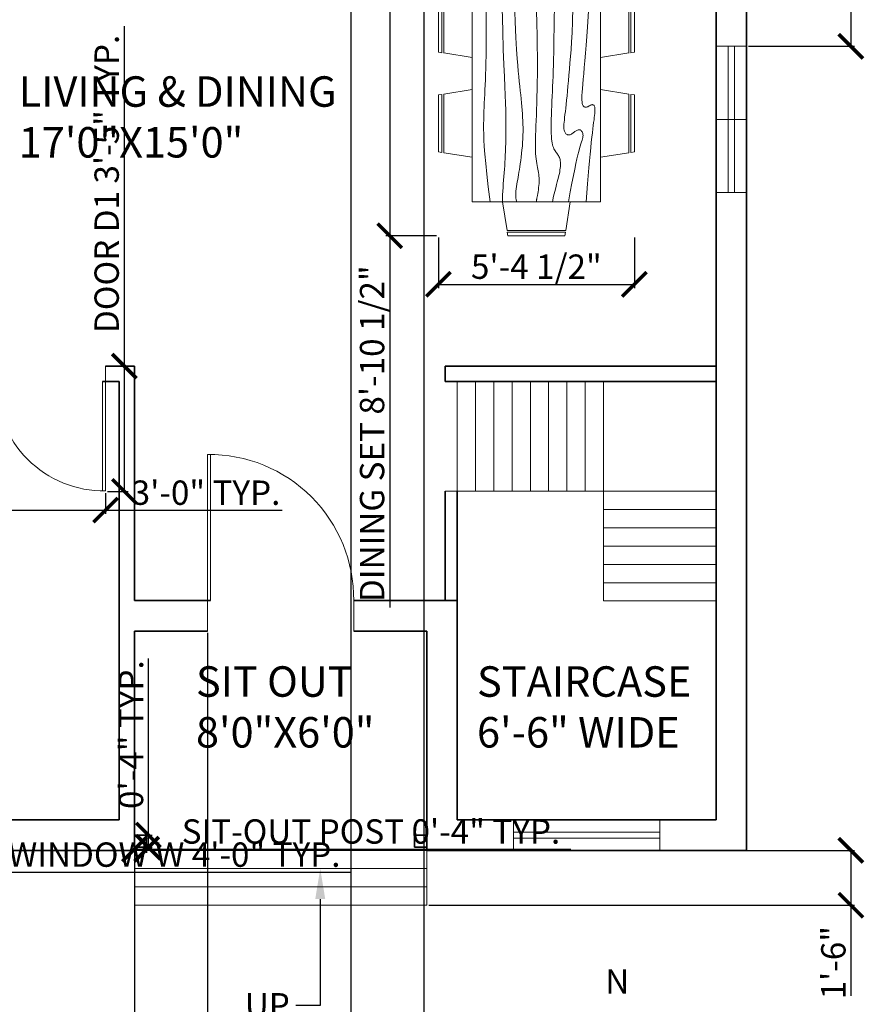
# Model space of a CAD drawing. Units: inches. Extents: x 21865 to 22885, y 36660 to 37408.
# Tile 3 of 6: x 22052 to 22329, y 36833 to 37157. Entities that reach past the tile are written whole.
import ezdxf
from ezdxf import colors
from ezdxf.entities.mleader import LeaderData, LeaderLine
from ezdxf.math import Vec2, Vec3

# ---------------------------------------------------------------- set-up
doc = ezdxf.new("R2010")
doc.units = ezdxf.units.IN
for name, color, linetype, lineweight in [('A-ANNO-DIMS', 2, 'Continuous', 18), ('A-ANNO-SYMB', 7, 'Continuous', 18), ('A-ANNO-TEXT', 7, 'Continuous', 18), ('A-AREA-IDEN', 7, 'Continuous', 20), ('A-COLS', 7, 'Continuous', 35), ('A-DOOR', 3, 'Continuous', 20), ('A-FLOR-STRS', 7, 'Continuous', 20), ('A-FURN', 8, 'Continuous', 18), ('A-GLAZ', 4, 'Continuous', 18), ('A-WALL', 7, 'Continuous', 35)]:
    doc.layers.add(name, color=color, linetype=linetype, lineweight=lineweight)
doc.styles.get("Standard").update_dxf_attribs({"font": 'arial.ttf'})
doc.dimstyles.new('ISO-25', dxfattribs={"dimtxt": 8, "dimasz": 8, "dimexe": 1.25, "dimexo": 0.625, "dimtad": 1, "dimlunit": 3, "dimtxsty": 'Standard', "dimblk": 'ARCHTICK', "dimcen": 2.5, "dimclrd": 4, "dimclre": 5, "dimclrt": 1, "dimadec": 0, "dimazin": 0, "dimtfac": 1, "dimtmove": 0, "dimatfit": 3, "dimfxl": 1, "dimarcsym": 0})

# ---------------------------------------------------------------- blocks, each defined once
blk = doc.blocks.new('Dining Set - 36 x 72 in.')
for p, q in [((-22.2343, 26.00059), (-23.4847, 17.99762)), ((-22.2304, 26), (-5.7608, 26)), ((-22, 27.5), (-22.1562, 26.50042)), ((-5.8416, 26.5), (-22.1534, 26.5)), ((-22, 27.5), (-6, 27.5)), ((-5.8437, 26.49966), (-6, 27.5)), ((-4.5152, 17.99762), (-5.7655, 25.99926)), ((5.7657, 26.00059), (4.5153, 17.99762)), ((5.7696, 26), (22.2392, 26)), ((6, 27.5), (5.8438, 26.50042)), ((22.1584, 26.5), (5.8466, 26.5)), ((6, 27.5), (22, 27.5)), ((22.1563, 26.49966), (22, 27.5)), ((23.4848, 17.99762), (22.2345, 25.99926)), ((36, 18), (-36, 18)), ((-36, 18), (-36, -18)), ((36, -18), (36, 18)), ((-44.0006, 8.23428), (-35.9976, 9.48474)), ((44.0006, 8.23428), (35.9976, 9.48474)), ((-45.5, 8), (-44.5004, 8.15617)), ((-45.5, 8), (-45.5, -8)), ((-44.5, -8.15843), (-44.5, 8.15338)), ((-44, 8.23041), (-44, -8.23915)), ((44, 8.23041), (44, -8.23915)), ((44.5, -8.15843), (44.5, 8.15338)), ((45.5, 8), (44.5005, 8.15617)), ((45.5, 8), (45.5, -8)), ((-44.4997, -8.15631), (-45.5, -8)), ((-35.9976, -9.48476), (-43.9993, -8.2345)), ((35.9976, -9.48476), (43.9993, -8.2345)), ((44.4997, -8.15631), (45.5, -8)), ((-36, -18), (36, -18)), ((-22.2343, -26.0006), (-23.4847, -17.99762)), ((-4.5152, -17.99762), (-5.7655, -25.99928)), ((5.7657, -26.0006), (4.5153, -17.99762)), ((23.4848, -17.99762), (22.2345, -25.99928)), ((-22.2304, -26), (-5.7608, -26)), ((-22, -27.5), (-22.1562, -26.50044)), ((-5.8416, -26.5), (-22.1534, -26.5)), ((-22, -27.5), (-6, -27.5)), ((-5.8437, -26.49967), (-6, -27.5)), ((5.7696, -26), (22.2392, -26)), ((6, -27.5), (5.8438, -26.50044)), ((22.1584, -26.5), (5.8466, -26.5)), ((6, -27.5), (22, -27.5)), ((22.1563, -26.49967), (22, -27.5))]:
    blk.add_line(p, q)
for points in [[(-36, 15), (-31.1772, 14.97754), (-26.8079, 14.91406), (-22.8538, 14.81543), (-19.276, 14.6875), (-16.0362, 14.53613), (-13.0957, 14.36718), (-10.4159, 14.18652), (-7.9583, 14), (-5.6904, 13.81315), (-3.6035, 13.63021), (-1.6954, 13.45508), (0.0365, 13.29166), (1.5945, 13.14388), (2.9811, 13.01562), (4.1988, 12.9108), (5.25, 12.83333), (6.1393, 12.78613), (6.8802, 12.76823), (7.4883, 12.77767), (7.9792, 12.8125), (8.3685, 12.87077), (8.6719, 12.95052), (8.9049, 13.0498), (9.0833, 13.16666), (9.2205, 13.29899), (9.3216, 13.44401), (9.3895, 13.59879), (9.4271, 13.76041), (9.4373, 13.92594), (9.4232, 14.09245), (9.3875, 14.257), (9.3333, 14.41666), (9.2638, 14.56917), (9.1836, 14.71484), (9.0975, 14.85465), (9.0104, 14.98958), (8.9272, 15.1206), (8.8529, 15.2487), (8.7922, 15.37483), (8.75, 15.5), (8.7305, 15.62467), (8.7344, 15.74739), (8.7617, 15.86621), (8.8125, 15.97916), (8.8867, 16.08431), (8.9844, 16.17968), (9.1055, 16.26334), (9.25, 16.33333), (9.4189, 16.38802), (9.6172, 16.42708), (9.8506, 16.45052), (10.125, 16.45833), (10.4463, 16.45052), (10.8203, 16.42708), (11.2529, 16.38802), (11.75, 16.33333), (12.3184, 16.26318), (12.9694, 16.17838), (13.7151, 16.07991), (14.5677, 15.96875), (15.5395, 15.84586), (16.6426, 15.71224), (17.8893, 15.56884), (19.2917, 15.41666), (20.859, 15.25667), (22.5879, 15.08984), (24.4721, 14.91715), (26.5052, 14.73958), (28.6809, 14.5581), (30.9929, 14.3737), (33.4347, 14.18733), (36, 14)], [(-36, 10), (-28.9766, 10.14274), (-23.1725, 10.20442), (-18.4241, 10.19775), (-14.5677, 10.13541), (-11.4399, 10.03011), (-8.877, 9.89453), (-6.7154, 9.74137), (-4.7917, 9.58333), (-2.9698, 9.43082), (-1.2246, 9.28515), (0.4415, 9.14534), (2.026, 9.01041), (3.5266, 8.87939), (4.9408, 8.7513), (6.266, 8.62516), (7.5, 8.5), (8.6411, 8.37549), (9.6914, 8.2539), (10.6538, 8.13818), (11.5312, 8.03125), (12.3267, 7.93603), (13.043, 7.85547), (13.6831, 7.79248), (14.25, 7.75), (14.7471, 7.7303), (15.1797, 7.73307), (15.5537, 7.75732), (15.875, 7.80208), (16.1494, 7.86637), (16.3828, 7.94922), (16.5811, 8.04964), (16.75, 8.16666), (16.8944, 8.29915), (17.0143, 8.44531), (17.1089, 8.60319), (17.1771, 8.77083), (17.218, 8.94629), (17.2305, 9.1276), (17.2137, 9.31282), (17.1667, 9.5), (17.0895, 9.6875), (16.987, 9.875), (16.8649, 10.0625), (16.7292, 10.25), (16.5856, 10.4375), (16.4401, 10.625), (16.2985, 10.8125), (16.1667, 11), (16.05, 11.18733), (15.9518, 11.3737), (15.8752, 11.5581), (15.8229, 11.73958), (15.798, 11.91715), (15.8034, 12.08984), (15.842, 12.25667), (15.9167, 12.41666), (16.0295, 12.56836), (16.1784, 12.70833), (16.3605, 12.83268), (16.5729, 12.9375), (16.8127, 13.01888), (17.0768, 13.07291), (17.3625, 13.0957), (17.6667, 13.08333), (17.9894, 13.03312), (18.3418, 12.94726), (18.7382, 12.82918), (19.1927, 12.68229), (19.7195, 12.51001), (20.3327, 12.31575), (21.0465, 12.10294), (21.875, 11.875), (22.8357, 11.63354), (23.959, 11.37304), (25.2786, 11.08618), (26.8282, 10.76562), (28.6414, 10.40405), (30.752, 9.99414), (33.1936, 9.52856), (36, 9)], [(-36, 5.5), (-30.7157, 5.3348), (-26.069, 5.20963), (-21.9946, 5.11767), (-18.4271, 5.05208), (-15.3009, 5.00602), (-12.5508, 4.97265), (-10.1112, 4.94515), (-7.9167, 4.91666), (-5.909, 4.88167), (-4.0586, 4.83984), (-2.3429, 4.79215), (-0.7396, 4.73958), (0.7739, 4.6831), (2.22, 4.6237), (3.6213, 4.56233), (5, 4.5), (6.373, 4.43782), (7.7344, 4.3776), (9.0723, 4.32129), (10.375, 4.27083), (11.6309, 4.22819), (12.8281, 4.19531), (13.9551, 4.17415), (15, 4.16666), (15.954, 4.17448), (16.819, 4.19791), (17.6001, 4.23698), (18.3021, 4.29166), (18.9299, 4.36198), (19.4883, 4.44791), (19.9823, 4.54948), (20.4167, 4.66666), (20.7969, 4.79899), (21.1302, 4.94401), (21.4245, 5.09879), (21.6875, 5.26041), (21.9271, 5.42594), (22.1511, 5.59245), (22.3672, 5.757), (22.5834, 5.91666), (22.8065, 6.06868), (23.0404, 6.21093), (23.2879, 6.34147), (23.5521, 6.45833), (23.8358, 6.55957), (24.142, 6.64323), (24.4735, 6.70735), (24.8334, 6.75), (25.2235, 6.76969), (25.642, 6.76692), (26.0858, 6.74267), (26.5521, 6.69791), (27.0379, 6.63362), (27.5404, 6.55078), (28.0565, 6.45036), (28.5834, 6.33333), (29.1242, 6.19987), (29.7071, 6.04687), (30.3661, 5.87044), (31.1354, 5.66666), (32.0493, 5.43164), (33.142, 5.16146), (34.4475, 4.85221), (36, 4.5)], [(-36, -1), (-30.7915, -0.6591), (-26.0195, -0.38216), (-21.6519, -0.16284), (-17.6563, 0.00521), (-14.0005, 0.12833), (-10.6523, 0.21289), (-7.5796, 0.26522), (-4.75, 0.29166), (-2.134, 0.29793), (0.2878, 0.28711), (2.5317, 0.26163), (4.6146, 0.22396), (6.5529, 0.17651), (8.3633, 0.12174), (10.0623, 0.06209), (11.6667, 0), (13.1899, -0.06201), (14.6341, -0.1211), (15.9982, -0.17432), (17.2813, -0.21875), (18.4823, -0.25147), (19.6003, -0.26953), (20.6343, -0.27002), (21.5834, -0.25), (22.4481, -0.20768), (23.2357, -0.14584), (23.9549, -0.06836), (24.6146, 0.02083), (25.2235, 0.11784), (25.7904, 0.21875), (26.3241, 0.31966), (26.8334, 0.41666), (27.3265, 0.50618), (27.8099, 0.58593), (28.2894, 0.65397), (28.7709, 0.70833), (29.2601, 0.74707), (29.763, 0.76823), (30.2855, 0.76985), (30.8334, 0.75), (31.4088, 0.70784), (31.9994, 0.64713), (32.589, 0.57275), (33.1615, 0.48958), (33.7008, 0.4025), (34.1908, 0.3164), (34.6153, 0.23616), (34.9584, 0.16666), (35.2099, 0.11165), (35.3848, 0.07031), (35.504, 0.04069), (35.5886, 0.02083), (35.6594, 0.00879), (35.7377, 0.0026), (35.8442, 0.00032), (36, 0)], [(-36, -6.5), (-27.1843, -6.31267), (-20.084, -6.1263), (-14.469, -5.9419), (-10.1094, -5.76042), (-6.7752, -5.58285), (-4.2363, -5.41016), (-2.2629, -5.24333), (-0.625, -5.08334), (0.8708, -4.93099), (2.2715, -4.78646), (3.5872, -4.64974), (4.8281, -4.52084), (6.0046, -4.39974), (7.127, -4.28646), (8.2053, -4.18099), (9.25, -4.08334), (10.2705, -3.99382), (11.2734, -3.91407), (12.2647, -3.84603), (13.25, -3.79167), (14.2354, -3.75293), (15.2266, -3.73177), (16.2295, -3.73015), (17.25, -3.75), (18.2912, -3.79248), (19.3451, -3.85547), (20.4009, -3.93604), (21.4479, -4.03125), (22.4754, -4.13819), (23.4727, -4.25391), (24.4289, -4.37549), (25.3334, -4.5), (26.1785, -4.62492), (26.9694, -4.74935), (27.7145, -4.87281), (28.4219, -4.99479), (29.1, -5.11483), (29.7572, -5.23242), (30.4016, -5.34709), (31.0417, -5.45834), (31.6837, -5.56437), (32.3262, -5.65821), (32.9658, -5.73153), (33.599, -5.77604), (34.2224, -5.78345), (34.8327, -5.74545), (35.4264, -5.65373), (36, -5.5)], [(-36, -10), (-26.4022, -9.81299), (-18.4675, -9.62891), (-11.9839, -9.45069), (-6.7396, -9.28125), (-2.5226, -9.12354), (0.8789, -8.98047), (3.6769, -8.85498), (6.0833, -8.75), (8.2767, -8.66765), (10.3021, -8.60677), (12.1712, -8.56543), (13.8958, -8.54167), (15.4876, -8.53353), (16.9583, -8.53907), (18.3197, -8.55632), (19.5834, -8.58334), (20.7616, -8.61841), (21.8685, -8.66081), (22.9188, -8.71004), (23.9271, -8.76563), (24.9081, -8.82707), (25.8763, -8.89388), (26.8465, -8.96558), (27.8334, -9.04167), (28.8474, -9.12118), (29.8828, -9.20117), (30.93, -9.27824), (31.9792, -9.34896), (33.0205, -9.40991), (34.0443, -9.45768), (35.0407, -9.48885), (36, -9.5)], [(-36, -14.5), (-30.0881, -14.33513), (-25.0332, -14.21224), (-20.7312, -14.12647), (-17.0781, -14.07292), (-13.97, -14.04671), (-11.3027, -14.04297), (-8.9724, -14.05681), (-6.875, -14.08334), (-4.9224, -14.11833), (-3.0905, -14.16016), (-1.3709, -14.20785), (0.2448, -14.26042), (1.7647, -14.3169), (3.1973, -14.3763), (4.5507, -14.43767), (5.8333, -14.5), (7.0554, -14.5621), (8.235, -14.62175), (9.3922, -14.67652), (10.5469, -14.72396), (11.7192, -14.76164), (12.929, -14.78711), (14.1965, -14.79794), (15.5417, -14.79167), (16.9933, -14.76424), (18.6152, -14.70508), (20.4804, -14.60197), (22.6615, -14.44271), (25.2312, -14.21509), (28.2624, -13.9069), (31.8277, -13.50594), (36, -13)]]:
    blk.add_lwpolyline(points)
blk = doc.blocks.new('WIN-W-48-PLAN')
for p, q in [((0, 0), (0, 10)), ((48, 0), (48, 10)), ((48, 6), (0, 6)), ((48, 4), (0, 4))]:
    blk.add_line(p, q)
blk = doc.blocks.new('DOOR-D1-36-PLAN')
for p, q in [((0, 36), (0, 41)), ((36, 36), (36, 41)), ((35, 36), (35, 0)), ((36, 36), (36, 0))]:
    blk.add_line(p, q)
blk.add_arc((35.5, 35.5), 35.5, 179.1931, 270.8069)
blk = doc.blocks.new('POST-SITOUT-4')
for p, q in [((4, 4), (0, 4)), ((4, 0), (4, 4)), ((0, 0), (2, 0)), ((2, 0), (4, 0))]:
    blk.add_line(p, q)
blk = doc.blocks.new('_ArchTick')
at = {"color": 0, "linetype": 'ByBlock', "const_width": 0.15}
blk.add_lwpolyline([(-0.5, -0.5), (0.5, 0.5)], dxfattribs=at)
blk = doc.blocks.new('*D30')
at = {"layer": 'A-ANNO-DIMS', "color": 5, "lineweight": -2, "transparency": 16777216}
for p, q in [((21988.43, 36883.31), (21988.43, 36875.48)), ((22036.43, 36883.31), (22036.43, 36875.48))]:
    blk.add_line(p, q, dxfattribs=at)
at = {"layer": 'A-ANNO-DIMS', "color": 4, "lineweight": -2, "transparency": 16777216}
for p, q in [((21988.43, 36876.73), (22036.43, 36876.73)), ((22036.43, 36876.73), (22160.57, 36876.73))]:
    blk.add_line(p, q, dxfattribs=at)
at = {"layer": 'Defpoints', "color": 0, "transparency": 16777216}
for p in [(21988.43, 36883.93), (22036.43, 36883.93), (22036.43, 36876.73)]:
    blk.add_point(p, dxfattribs=at)
at = {"layer": 'A-ANNO-DIMS', "color": 4, "lineweight": -2, "transparency": 16777216, "xscale": 8, "yscale": 8, "zscale": 8, "rotation": 180}
blk.add_blockref('_ArchTick', (21988.43, 36876.73), dxfattribs=at)
at = {"layer": 'A-ANNO-DIMS', "color": 4, "lineweight": -2, "transparency": 16777216, "xscale": 8, "yscale": 8, "zscale": 8}
blk.add_blockref('_ArchTick', (22036.43, 36876.73), dxfattribs=at)
at = {"layer": 'A-ANNO-DIMS', "color": 1, "transparency": 16777216, "insert": (22102.5, 36881.5), "char_height": 8, "attachment_point": 5}
blk.add_mtext('WINDOW W 4\'-0" TYP.', dxfattribs=at)
blk = doc.blocks.new('*D36')
at = {"layer": 'A-ANNO-DIMS', "color": 4, "lineweight": -2, "transparency": 16777216}
for p, q in [((22086.1, 37042.93), (22086.1, 37154.57)), ((22086.1, 37001.8), (22086.1, 37042.93))]:
    blk.add_line(p, q, dxfattribs=at)
at = {"layer": 'A-ANNO-DIMS', "color": 5, "lineweight": -2, "transparency": 16777216}
for p, q in [((22080.55, 37042.93), (22087.35, 37042.93)), ((22080.55, 37001.8), (22087.35, 37001.8))]:
    blk.add_line(p, q, dxfattribs=at)
at = {"layer": 'Defpoints', "color": 0, "transparency": 16777216}
for p in [(22079.93, 37042.93), (22086.1, 37042.93), (22079.93, 37001.8)]:
    blk.add_point(p, dxfattribs=at)
at = {"layer": 'A-ANNO-DIMS', "color": 4, "lineweight": -2, "transparency": 16777216, "xscale": 8, "yscale": 8, "zscale": 8}
for p, rotation in [((22086.1, 37042.93), 90), ((22086.1, 37001.8), 270)]:
    blk.add_blockref('_ArchTick', p, dxfattribs=dict(at, rotation=rotation))
at = {"layer": 'A-ANNO-DIMS', "color": 1, "transparency": 16777216, "insert": (22081.33, 37102.75), "char_height": 8, "attachment_point": 5, "rotation": 90}
blk.add_mtext('DOOR D1 3\'-5" TYP.', dxfattribs=at)
blk = doc.blocks.new('*D37')
at = {"layer": 'A-ANNO-DIMS', "color": 5, "lineweight": -2, "transparency": 16777216}
for p, q in [((22043.79, 37001.17), (22043.79, 36994.38)), ((22079.93, 37001.17), (22079.93, 36994.38))]:
    blk.add_line(p, q, dxfattribs=at)
at = {"layer": 'A-ANNO-DIMS', "color": 4, "lineweight": -2, "transparency": 16777216}
for p, q in [((22043.79, 36995.63), (22079.93, 36995.63)), ((22079.93, 36995.63), (22137.94, 36995.63))]:
    blk.add_line(p, q, dxfattribs=at)
at = {"layer": 'Defpoints', "color": 0, "transparency": 16777216}
for p in [(22043.79, 37001.8), (22079.93, 37001.8), (22079.93, 36995.63)]:
    blk.add_point(p, dxfattribs=at)
at = {"layer": 'A-ANNO-DIMS', "color": 4, "lineweight": -2, "transparency": 16777216, "xscale": 8, "yscale": 8, "zscale": 8, "rotation": 180}
blk.add_blockref('_ArchTick', (22043.79, 36995.63), dxfattribs=at)
at = {"layer": 'A-ANNO-DIMS', "color": 4, "lineweight": -2, "transparency": 16777216, "xscale": 8, "yscale": 8, "zscale": 8}
blk.add_blockref('_ArchTick', (22079.93, 36995.63), dxfattribs=at)
at = {"layer": 'A-ANNO-DIMS', "color": 1, "transparency": 16777216, "insert": (22112.93, 37000.34), "char_height": 8, "attachment_point": 5}
blk.add_mtext('3\'-0" TYP.', dxfattribs=at)
blk = doc.blocks.new('*D38')
at = {"layer": 'A-ANNO-DIMS', "color": 4, "lineweight": -2, "transparency": 16777216}
for p, q in [((22089.43, 36884.34), (22093.43, 36884.34)), ((22093.43, 36884.34), (22232.74, 36884.34))]:
    blk.add_line(p, q, dxfattribs=at)
at = {"layer": 'A-ANNO-DIMS', "color": 5, "lineweight": -2, "transparency": 16777216}
for p, q in [((22089.43, 36884.31), (22089.43, 36883.09)), ((22093.43, 36884.31), (22093.43, 36883.09))]:
    blk.add_line(p, q, dxfattribs=at)
at = {"layer": 'Defpoints', "color": 0, "transparency": 16777216}
for p in [(22089.43, 36884.94), (22093.43, 36884.94), (22093.43, 36884.34)]:
    blk.add_point(p, dxfattribs=at)
at = {"layer": 'A-ANNO-DIMS', "color": 4, "lineweight": -2, "transparency": 16777216, "xscale": 8, "yscale": 8, "zscale": 8, "rotation": 180}
blk.add_blockref('_ArchTick', (22089.43, 36884.34), dxfattribs=at)
at = {"layer": 'A-ANNO-DIMS', "color": 4, "lineweight": -2, "transparency": 16777216, "xscale": 8, "yscale": 8, "zscale": 8}
blk.add_blockref('_ArchTick', (22093.43, 36884.34), dxfattribs=at)
at = {"layer": 'A-ANNO-DIMS', "color": 1, "transparency": 16777216, "insert": (22167.09, 36889.1), "char_height": 8, "attachment_point": 5}
blk.add_mtext('SIT-OUT POST 0\'-4" TYP.', dxfattribs=at)
blk = doc.blocks.new('*D39')
at = {"layer": 'A-ANNO-DIMS', "color": 4, "lineweight": -2, "transparency": 16777216}
for p, q in [((22094.03, 36888.94), (22094.03, 36946.95)), ((22094.03, 36884.94), (22094.03, 36888.94))]:
    blk.add_line(p, q, dxfattribs=at)
at = {"layer": 'A-ANNO-DIMS', "color": 5, "lineweight": -2, "transparency": 16777216}
for p, q in [((22094.05, 36888.94), (22095.28, 36888.94)), ((22094.05, 36884.94), (22095.28, 36884.94))]:
    blk.add_line(p, q, dxfattribs=at)
at = {"layer": 'Defpoints', "color": 0, "transparency": 16777216}
for p in [(22093.43, 36888.94), (22094.03, 36888.94), (22093.43, 36884.94)]:
    blk.add_point(p, dxfattribs=at)
at = {"layer": 'A-ANNO-DIMS', "color": 4, "lineweight": -2, "transparency": 16777216, "xscale": 8, "yscale": 8, "zscale": 8}
for p, rotation in [((22094.03, 36888.94), 90), ((22094.03, 36884.94), 270)]:
    blk.add_blockref('_ArchTick', p, dxfattribs=dict(at, rotation=rotation))
at = {"layer": 'A-ANNO-DIMS', "color": 1, "transparency": 16777216, "insert": (22089.32, 36921.94), "char_height": 8, "attachment_point": 5, "rotation": 90}
blk.add_mtext('0\'-4" TYP.', dxfattribs=at)
blk = doc.blocks.new('*D48')
at = {"layer": 'A-ANNO-DIMS', "color": 5, "lineweight": -2, "transparency": 16777216}
for p, q in [((22188.6, 37192.23), (22172.01, 37192.23)), ((22188.6, 37085.76), (22172.01, 37085.76))]:
    blk.add_line(p, q, dxfattribs=at)
at = {"layer": 'A-ANNO-DIMS', "color": 4, "lineweight": -2, "transparency": 16777216}
for p, q in [((22173.26, 37192.23), (22173.26, 37085.76)), ((22173.26, 37085.76), (22173.26, 36963.72))]:
    blk.add_line(p, q, dxfattribs=at)
at = {"layer": 'Defpoints', "color": 0, "transparency": 16777216}
for p in [(22189.23, 37192.23), (22173.26, 37085.76), (22189.23, 37085.76)]:
    blk.add_point(p, dxfattribs=at)
at = {"layer": 'A-ANNO-DIMS', "color": 4, "lineweight": -2, "transparency": 16777216, "xscale": 8, "yscale": 8, "zscale": 8}
for p, rotation in [((22173.26, 37192.23), 90), ((22173.26, 37085.76), 270)]:
    blk.add_blockref('_ArchTick', p, dxfattribs=dict(at, rotation=rotation))
at = {"layer": 'A-ANNO-DIMS', "color": 1, "transparency": 16777216, "insert": (22168.49, 37020.74), "char_height": 8, "attachment_point": 5, "rotation": 90}
blk.add_mtext('DINING SET 8\'-10 1/2"', dxfattribs=at)
blk = doc.blocks.new('*D49')
at = {"layer": 'A-ANNO-DIMS', "color": 5, "lineweight": -2, "transparency": 16777216}
for p, q in [((22189.23, 37085.13), (22189.23, 37068.53)), ((22253.58, 37085.13), (22253.58, 37068.53))]:
    blk.add_line(p, q, dxfattribs=at)
at = {"layer": 'A-ANNO-DIMS', "color": 4, "lineweight": -2, "transparency": 16777216}
blk.add_line((22189.23, 37069.78), (22253.58, 37069.78), dxfattribs=at)
at = {"layer": 'Defpoints', "color": 0, "transparency": 16777216}
for p in [(22189.23, 37085.76), (22253.58, 37085.76), (22253.58, 37069.78)]:
    blk.add_point(p, dxfattribs=at)
at = {"layer": 'A-ANNO-DIMS', "color": 4, "lineweight": -2, "transparency": 16777216, "xscale": 8, "yscale": 8, "zscale": 8, "rotation": 180}
blk.add_blockref('_ArchTick', (22189.23, 37069.78), dxfattribs=at)
at = {"layer": 'A-ANNO-DIMS', "color": 4, "lineweight": -2, "transparency": 16777216, "xscale": 8, "yscale": 8, "zscale": 8}
blk.add_blockref('_ArchTick', (22253.58, 37069.78), dxfattribs=at)
at = {"layer": 'A-ANNO-DIMS', "color": 1, "transparency": 16777216, "insert": (22221.4, 37074.55), "char_height": 8, "attachment_point": 5}
blk.add_mtext('5\'-4 1/2"', dxfattribs=at)
blk = doc.blocks.new('*D57')
at = {"layer": 'A-ANNO-DIMS', "color": 5, "lineweight": -2, "transparency": 16777216}
for p, q in [((22291.05, 37269.93), (22325.93, 37269.93)), ((22291.05, 37147.93), (22325.93, 37147.93))]:
    blk.add_line(p, q, dxfattribs=at)
at = {"layer": 'A-ANNO-DIMS', "color": 4, "lineweight": -2, "transparency": 16777216}
blk.add_line((22324.68, 37269.93), (22324.68, 37147.93), dxfattribs=at)
at = {"layer": 'Defpoints', "color": 0, "transparency": 16777216}
for p in [(22290.43, 37269.93), (22290.43, 37147.93), (22324.68, 37147.93)]:
    blk.add_point(p, dxfattribs=at)
at = {"layer": 'A-ANNO-DIMS', "color": 4, "lineweight": -2, "transparency": 16777216, "xscale": 8, "yscale": 8, "zscale": 8}
for p, rotation in [((22324.68, 37269.93), 90), ((22324.68, 37147.93), 270)]:
    blk.add_blockref('_ArchTick', p, dxfattribs=dict(at, rotation=rotation))
at = {"layer": 'A-ANNO-DIMS', "color": 1, "transparency": 16777216, "insert": (22319.97, 37208.93), "char_height": 8, "attachment_point": 5, "rotation": 90}
blk.add_mtext('10\'-2"', dxfattribs=at)
blk = doc.blocks.new('*D58')
at = {"layer": 'A-ANNO-DIMS', "color": 5, "lineweight": -2, "transparency": 16777216}
for p, q in [((22160.43, 37233.31), (22160.43, 36662.83)), ((22184.43, 37233.31), (22184.43, 36662.83))]:
    blk.add_line(p, q, dxfattribs=at)
at = {"layer": 'A-ANNO-DIMS', "color": 4, "lineweight": -2, "transparency": 16777216}
blk.add_line((22160.43, 36664.08), (22184.43, 36664.08), dxfattribs=at)
at = {"layer": 'Defpoints', "color": 0, "transparency": 16777216}
for p in [(22160.43, 37233.93), (22184.43, 37233.93), (22184.43, 36664.08)]:
    blk.add_point(p, dxfattribs=at)
at = {"layer": 'A-ANNO-DIMS', "color": 4, "lineweight": -2, "transparency": 16777216, "xscale": 8, "yscale": 8, "zscale": 8, "rotation": 180}
blk.add_blockref('_ArchTick', (22160.43, 36664.08), dxfattribs=at)
at = {"layer": 'A-ANNO-DIMS', "color": 4, "lineweight": -2, "transparency": 16777216, "xscale": 8, "yscale": 8, "zscale": 8}
blk.add_blockref('_ArchTick', (22184.43, 36664.08), dxfattribs=at)
at = {"layer": 'A-ANNO-DIMS', "color": 1, "transparency": 16777216, "insert": (22172.43, 36668.79), "char_height": 8, "attachment_point": 5}
blk.add_mtext('2\'-0"', dxfattribs=at)
blk = doc.blocks.new('*D59')
at = {"layer": 'A-ANNO-DIMS', "color": 5, "lineweight": -2, "transparency": 16777216}
for p, q in [((22089.43, 36955.31), (22089.43, 36662.83)), ((22113.43, 36955.31), (22113.43, 36662.83))]:
    blk.add_line(p, q, dxfattribs=at)
at = {"layer": 'A-ANNO-DIMS', "color": 4, "lineweight": -2, "transparency": 16777216}
blk.add_line((22089.43, 36664.08), (22113.43, 36664.08), dxfattribs=at)
at = {"layer": 'Defpoints', "color": 0, "transparency": 16777216}
for p in [(22089.43, 36955.93), (22113.43, 36955.93), (22113.43, 36664.08)]:
    blk.add_point(p, dxfattribs=at)
at = {"layer": 'A-ANNO-DIMS', "color": 4, "lineweight": -2, "transparency": 16777216, "xscale": 8, "yscale": 8, "zscale": 8, "rotation": 180}
blk.add_blockref('_ArchTick', (22089.43, 36664.08), dxfattribs=at)
at = {"layer": 'A-ANNO-DIMS', "color": 4, "lineweight": -2, "transparency": 16777216, "xscale": 8, "yscale": 8, "zscale": 8}
blk.add_blockref('_ArchTick', (22113.43, 36664.08), dxfattribs=at)
at = {"layer": 'A-ANNO-DIMS', "color": 1, "transparency": 16777216, "insert": (22101.43, 36668.79), "char_height": 8, "attachment_point": 5}
blk.add_mtext('2\'-0"', dxfattribs=at)
blk = doc.blocks.new('*D60')
at = {"layer": 'A-ANNO-DIMS', "color": 5, "lineweight": -2, "transparency": 16777216}
for p, q in [((22186.05, 36883.93), (22325.93, 36883.93)), ((22186.05, 36865.93), (22325.93, 36865.93))]:
    blk.add_line(p, q, dxfattribs=at)
at = {"layer": 'A-ANNO-DIMS', "color": 4, "lineweight": -2, "transparency": 16777216}
for p, q in [((22324.68, 36883.93), (22324.68, 36865.93)), ((22324.68, 36865.93), (22324.68, 36836.17))]:
    blk.add_line(p, q, dxfattribs=at)
at = {"layer": 'Defpoints', "color": 0, "transparency": 16777216}
for p in [(22185.43, 36883.93), (22185.43, 36865.93), (22324.68, 36865.93)]:
    blk.add_point(p, dxfattribs=at)
at = {"layer": 'A-ANNO-DIMS', "color": 4, "lineweight": -2, "transparency": 16777216, "xscale": 8, "yscale": 8, "zscale": 8}
for p, rotation in [((22324.68, 36883.93), 90), ((22324.68, 36865.93), 270)]:
    blk.add_blockref('_ArchTick', p, dxfattribs=dict(at, rotation=rotation))
at = {"layer": 'A-ANNO-DIMS', "color": 1, "transparency": 16777216, "insert": (22319.97, 36847.05), "char_height": 8, "attachment_point": 5, "rotation": 90}
blk.add_mtext('1\'-6"', dxfattribs=at)

msp = doc.modelspace()

# ---------------------------------------------------------------- linework, layer by layer
at = {"layer": 'A-DOOR'}
for p, q in [((22113.43, 36965.931), (22113.43, 37013.931)), ((22114.43, 36965.931), (22114.43, 37013.931)), ((22113.43, 36955.931), (22113.43, 36965.931)), ((22161.43, 36955.931), (22161.43, 36965.931)), ((22161.43, 36965.931), (22161.43, 36965.931))]:
    msp.add_line(p, q, dxfattribs=at)
msp.add_arc((22113.93, 36966.431), 47.503, 359.39691, 90.60309, dxfattribs=at)
at = {"layer": 'A-FLOR-STRS'}
for p, q in [((22195.43, 37001.826), (22195.43, 37037.931)), ((22201.43, 37001.826), (22201.43, 37037.931)), ((22207.43, 37001.826), (22207.43, 37037.931)), ((22213.43, 37001.826), (22213.43, 37037.931)), ((22219.43, 37001.826), (22219.43, 37037.931)), ((22225.43, 37001.826), (22225.43, 37037.931)), ((22231.43, 37001.826), (22231.43, 37037.931)), ((22237.43, 37001.826), (22237.43, 37037.931)), ((22243.43, 37001.826), (22243.43, 37037.931)), ((22191.43, 37001.826), (22280.43, 37001.826)), ((22243.43, 37001.826), (22243.43, 36965.826)), ((22243.43, 36995.826), (22280.43, 36995.826)), ((22243.43, 36989.826), (22280.43, 36989.826)), ((22243.43, 36983.826), (22280.43, 36983.826)), ((22243.43, 36977.826), (22280.43, 36977.826)), ((22243.43, 36971.826), (22280.43, 36971.826)), ((22243.43, 36965.826), (22280.43, 36965.826)), ((22089.43, 36883.931), (22185.43, 36883.931)), ((22089.43, 36883.931), (22089.43, 36865.931)), ((22185.43, 36883.931), (22185.43, 36865.931)), ((22089.43, 36877.931), (22185.43, 36877.931)), ((22089.43, 36871.931), (22185.43, 36871.931)), ((22089.43, 36865.931), (22185.43, 36865.931))]:
    msp.add_line(p, q, dxfattribs=at)
at = {"layer": 'A-GLAZ'}
msp.add_line((22290.43, 37123.931), (22280.43, 37123.931), dxfattribs=at)
at = {"layer": 'A-WALL'}
for p, q in [((22290.43, 37363.931), (22290.43, 36883.931)), ((22280.43, 37229.931), (22280.43, 36893.931)), ((22089.43, 37042.931), (22079.93, 37042.931)), ((22089.43, 36965.931), (22089.43, 37042.931)), ((22280.43, 37042.931), (22191.43, 37042.931)), ((22191.43, 37037.931), (22191.43, 37042.931)), ((22084.43, 37037.931), (22078.93, 37037.931)), ((22084.43, 37037.931), (22078.93, 37037.931)), ((22084.43, 36893.931), (22084.43, 37037.931)), ((22280.43, 37037.931), (22191.43, 37037.931)), ((22191.43, 36965.931), (22191.43, 37001.826)), ((22191.43, 36965.931), (22191.43, 37001.826)), ((22195.43, 36975.931), (22195.43, 37001.826)), ((22195.43, 36893.931), (22195.43, 36975.931)), ((22114.43, 36965.931), (22089.43, 36965.931)), ((22195.43, 36965.931), (22161.43, 36965.931)), ((22089.43, 36883.931), (22089.43, 36955.931)), ((22113.43, 36955.931), (22089.43, 36955.931)), ((22185.43, 36955.931), (22161.43, 36955.931)), ((22185.43, 36883.931), (22185.43, 36955.931)), ((22084.43, 36893.931), (21940.43, 36893.931)), ((22280.43, 36893.931), (22195.43, 36893.931)), ((22089.43, 36883.931), (21930.43, 36883.931)), ((22290.43, 36883.931), (22185.43, 36883.931))]:
    msp.add_line(p, q, dxfattribs=at)

# ---------------------------------------------------------------- block references
at = {"layer": 'A-COLS'}
msp.add_blockref('POST-SITOUT-4', (22089.43, 36884.938), dxfattribs=at)
at = {"layer": 'A-COLS', "extrusion": (0, 0, -1), "zscale": -1}
msp.add_blockref('POST-SITOUT-4', (-22185.43, 36884.938), dxfattribs=at)
at = {"layer": 'A-DOOR'}
msp.add_blockref('DOOR-D1-36-PLAN', (22043.929, 37001.93), dxfattribs=at)
at = {"layer": 'A-FURN', "xscale": 1.170096591713225, "yscale": 1.170096591713225, "zscale": 1.170096591713225, "rotation": 270}
msp.add_blockref('Dining Set - 36 x 72 in.', (22221.405, 37138.995), dxfattribs=at)
at = {"layer": 'A-GLAZ', "rotation": 269.9999999999834}
msp.add_blockref('WIN-W-48-PLAN', (22280.429, 37147.931), dxfattribs=at)
at = {"layer": 'A-GLAZ'}
msp.add_blockref('WIN-W-48-PLAN', (22213.93, 36883.931), dxfattribs=at)

# ---------------------------------------------------------------- texts
at = {"layer": 'A-ANNO-SYMB', "insert": (22244.029, 36844.925), "char_height": 8, "width": 22.941, "attachment_point": 1}
msp.add_mtext('N', dxfattribs=at)
at = {"layer": 'A-AREA-IDEN', "char_height": 10, "attachment_point": 1}
for s, insert in [('LIVING & DINING\\P17\'0"X15\'0"', (22051.413, 37138.084)), ('SIT OUT\\P8\'0"X6\'0"', (22109.619, 36944.369)), ('STAIRCASE\\P6\'-6" WIDE', (22201.911, 36944.369))]:
    msp.add_mtext_dynamic_manual_height_columns(s, width=146.69061, gutter_width=12.5, heights=[0], dxfattribs=dict(at, insert=insert))

# ---------------------------------------------------------------- dimensions: what is measured, and where the dimension line sits
at = {"layer": 'A-ANNO-DIMS'}
for base, p1, p2, picture, middle in [((22324.68, 37147.931), (22290.43, 37269.931), (22290.43, 37147.931), '*D57', (22319.97, 37208.931)), ((22324.68, 36865.931), (22185.43, 36883.931), (22185.43, 36865.931), '*D60', (22319.97, 36847.05))]:
    dim = msp.add_linear_dim(base=base, p1=p1, p2=p2, angle=90, dimstyle='ISO-25', override={"dimdec": 1, "dimlfac": 1, "dimrnd": 0, "dimzin": 1, "dimdsep": 46, "dimlunit": 4, "dimfrac": 2}, dxfattribs=at)
    dim.commit()
    dim.dimension.update_dxf_attribs({"geometry": picture, "text_midpoint": middle})
for base, p1, p2, picture, middle in [((22184.43, 36664.077), (22160.43, 37233.931), (22184.43, 37233.931), '*D58', (22172.43, 36668.787)), ((22253.582, 37069.784), (22189.227, 37085.755), (22253.582, 37085.755), '*D49', (22221.405, 37074.545)), ((22113.43, 36664.077), (22089.43, 36955.931), (22113.43, 36955.931), '*D59', (22101.43, 36668.787))]:
    dim = msp.add_linear_dim(base=base, p1=p1, p2=p2, dimstyle='ISO-25', override={"dimdec": 1, "dimlfac": 1, "dimrnd": 0, "dimzin": 1, "dimdsep": 46, "dimlunit": 4, "dimfrac": 2}, dxfattribs=at)
    dim.commit()
    dim.dimension.update_dxf_attribs({"geometry": picture, "text_midpoint": middle})
for base, p1, p2, angle, text, picture, middle in [((22173.255, 37085.755), (22189.227, 37192.234), (22189.227, 37085.755), 270, 'DINING SET <>', '*D48', (22168.494, 37020.738)), ((22086.1, 37042.931), (22079.93, 37001.796), (22079.93, 37042.931), 90, 'DOOR D1 <> TYP.', '*D36', (22081.333, 37102.751)), ((22094.03, 36888.938), (22093.43, 36884.938), (22093.43, 36888.938), 90, '<> TYP.', '*D39', (22089.32, 36921.945))]:
    dim = msp.add_linear_dim(base=base, p1=p1, p2=p2, angle=angle, text=text, dimstyle='ISO-25', override={"dimdec": 1, "dimlfac": 1, "dimrnd": 0, "dimzin": 1, "dimdsep": 46, "dimlunit": 4, "dimfrac": 2}, dxfattribs=at)
    dim.commit()
    dim.dimension.update_dxf_attribs({"geometry": picture, "text_midpoint": middle})
for base, p1, p2, text, picture, middle in [((22079.93, 36995.626), (22043.795, 37001.796), (22079.93, 37001.796), '<> TYP.', '*D37', (22112.934, 37000.338)), ((22093.43, 36884.338), (22089.43, 36884.938), (22093.43, 36884.938), 'SIT-OUT POST <> TYP.', '*D38', (22167.086, 36889.102)), ((22036.43, 36876.731), (21988.43, 36883.931), (22036.43, 36883.931), 'WINDOW W <> TYP.', '*D30', (22102.498, 36881.496))]:
    dim = msp.add_linear_dim(base=base, p1=p1, p2=p2, text=text, dimstyle='ISO-25', override={"dimdec": 1, "dimlfac": 1, "dimrnd": 0, "dimzin": 1, "dimdsep": 46, "dimlunit": 4, "dimfrac": 2}, dxfattribs=at)
    dim.commit()
    dim.dimension.update_dxf_attribs({"geometry": picture, "text_midpoint": middle})

# ---------------------------------------------------------------- leaders
at = {"layer": 'A-ANNO-TEXT'}
ml = msp.add_multileader_mtext('Standard', dxfattribs=at)
ml.set_content('UP', color=256)
ml.set_leader_properties()
ml.build(insert=Vec2(0, 0))
ml.multileader.update_dxf_attribs({"arrow_head_size": 10})
ctx = ml.context
ctx.base_point, ctx.char_height, ctx.arrow_head_size, ctx.plane_origin = Vec3(22124.274, 36832.999), 8, 10, Vec3(22150.435, 36877.931)
ctx.text_align_type = 2
notes = []
notes.append((ctx, [(0, (1, 1, 0), (22150.435, 36832.999), (-1, 0), 8, [(0, [(22150.435, 36877.931)], 0, [])])]))
ctx.mtext.insert, ctx.mtext.alignment, ctx.mtext.flow_direction = Vec3(22140.435, 36837.068), 3, 5
for ctx, leaders in notes:
    for number, flags, end, landing, length, lines in leaders:
        leader = LeaderData()
        leader.index, (leader.has_last_leader_line, leader.has_dogleg_vector, leader.attachment_direction) = number, flags
        leader.last_leader_point, leader.dogleg_vector, leader.dogleg_length = Vec3(end), Vec3(landing), length
        for number, points, colour, breaks in lines:
            line = LeaderLine()
            line.index, line.vertices, line.color, line.breaks = number, Vec3.list(points), colors.encode_raw_color(colour), breaks
            leader.lines.append(line)
        ctx.leaders.append(leader)

doc.saveas('drawing.dxf')
